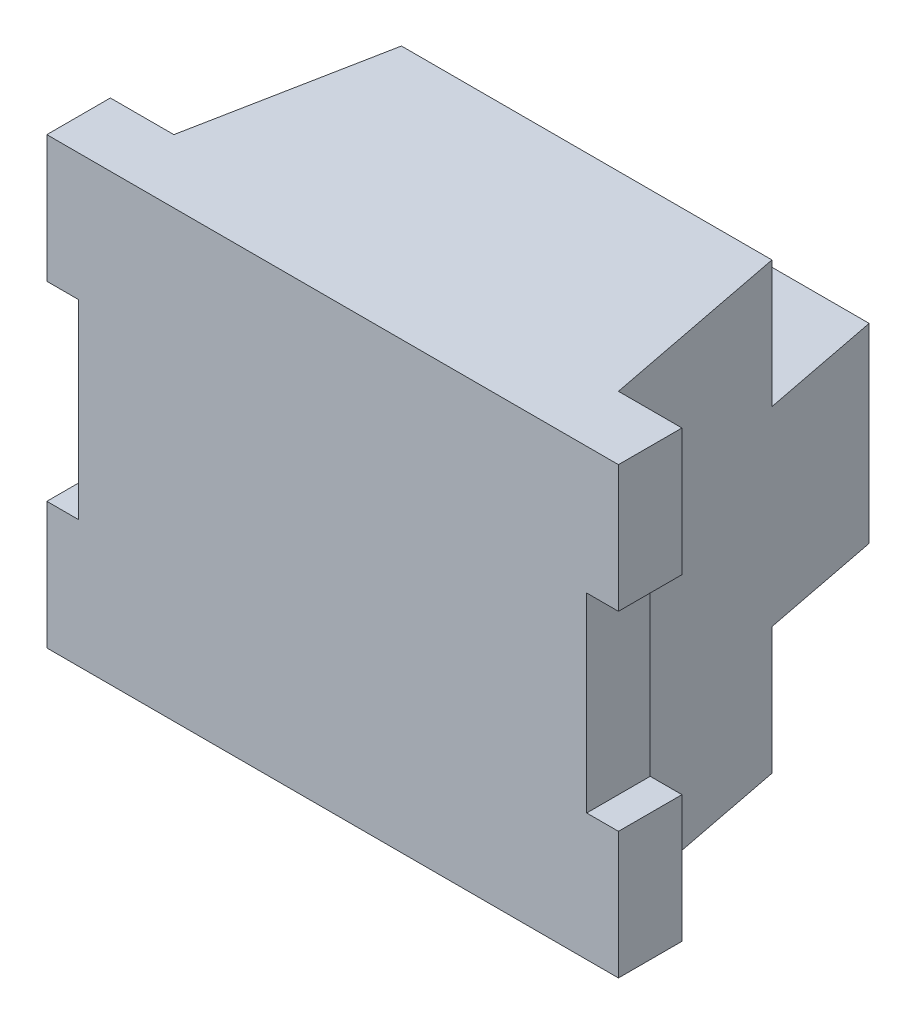
ISO-10303-21;
HEADER;
FILE_DESCRIPTION(('STEP AP214'),'2;1');
FILE_NAME('part.step','',(''),(''),'','','');
FILE_SCHEMA(('AUTOMOTIVE_DESIGN { 1 0 10303 214 1 1 1 1 }'));
ENDSEC;
DATA;
#1=APPLICATION_CONTEXT('core data for automotive mechanical design processes');
#2=APPLICATION_PROTOCOL_DEFINITION('international standard','automotive_design',2000,#1);
#3=PRODUCT_CONTEXT('',#1,'mechanical');
#4=PRODUCT('Part','Part','',(#3));
#5=PRODUCT_RELATED_PRODUCT_CATEGORY('part','',(#4));
#6=PRODUCT_DEFINITION_FORMATION('','',#4);
#7=PRODUCT_DEFINITION_CONTEXT('part definition',#1,'design');
#8=PRODUCT_DEFINITION('design','',#6,#7);
#9=PRODUCT_DEFINITION_SHAPE('','',#8);
#10=(LENGTH_UNIT() NAMED_UNIT(*) SI_UNIT(.MILLI.,.METRE.));
#11=(NAMED_UNIT(*) PLANE_ANGLE_UNIT() SI_UNIT($,.RADIAN.));
#12=(NAMED_UNIT(*) SI_UNIT($,.STERADIAN.) SOLID_ANGLE_UNIT());
#13=UNCERTAINTY_MEASURE_WITH_UNIT(LENGTH_MEASURE(1.E-05),#10,'distance_accuracy_value','');
#14=(GEOMETRIC_REPRESENTATION_CONTEXT(3) GLOBAL_UNCERTAINTY_ASSIGNED_CONTEXT((#13)) GLOBAL_UNIT_ASSIGNED_CONTEXT((#10,
#11,#12)) REPRESENTATION_CONTEXT('',''));
#15=CARTESIAN_POINT('',(0.,0.,0.));
#16=DIRECTION('',(0.,0.,1.));
#17=DIRECTION('',(1.,0.,0.));
#18=AXIS2_PLACEMENT_3D('',#15,#16,#17);
#19=CARTESIAN_POINT('',(-45.,35.,10.));
#20=DIRECTION('',(0.,-1.,0.));
#21=DIRECTION('',(0.,0.,-1.));
#22=AXIS2_PLACEMENT_3D('',#19,#20,#21);
#23=PLANE('',#22);
#24=DIRECTION('',(1.,0.,0.));
#25=VECTOR('',#24,1.);
#26=CARTESIAN_POINT('',(38.9138217050319,35.,-30.));
#27=LINE('',#26,#25);
#28=CARTESIAN_POINT('',(-29.1685907258683,35.,-30.));
#29=VERTEX_POINT('',#28);
#30=CARTESIAN_POINT('',(29.1685907258683,35.,-30.));
#31=VERTEX_POINT('',#30);
#32=EDGE_CURVE('E61',#29,#31,#27,.T.);
#33=ORIENTED_EDGE('',*,*,#32,.F.);
#34=DIRECTION('',(-0.190808995376549,0.,0.981627183447663));
#35=VECTOR('',#34,1.);
#36=CARTESIAN_POINT('',(-25.4753648522516,35.,-49.));
#37=LINE('',#36,#35);
#38=CARTESIAN_POINT('',(-35.,35.,0.));
#39=VERTEX_POINT('',#38);
#40=EDGE_CURVE('E209',#29,#39,#37,.T.);
#41=ORIENTED_EDGE('',*,*,#40,.T.);
#42=DIRECTION('',(-1.,0.,0.));
#43=VECTOR('',#42,1.);
#44=CARTESIAN_POINT('',(-45.,35.,0.));
#45=LINE('',#44,#43);
#46=CARTESIAN_POINT('',(-45.,35.,0.));
#47=VERTEX_POINT('',#46);
#48=EDGE_CURVE('E259',#39,#47,#45,.T.);
#49=ORIENTED_EDGE('',*,*,#48,.T.);
#50=DIRECTION('',(0.,0.,-1.));
#51=VECTOR('',#50,1.);
#52=CARTESIAN_POINT('',(-45.,35.,10.));
#53=LINE('',#52,#51);
#54=CARTESIAN_POINT('',(-45.,35.,10.));
#55=VERTEX_POINT('',#54);
#56=EDGE_CURVE('E291',#55,#47,#53,.T.);
#57=ORIENTED_EDGE('',*,*,#56,.F.);
#58=DIRECTION('',(-1.,0.,0.));
#59=VECTOR('',#58,1.);
#60=CARTESIAN_POINT('',(-45.,35.,10.));
#61=LINE('',#60,#59);
#62=CARTESIAN_POINT('',(45.,35.,10.));
#63=VERTEX_POINT('',#62);
#64=EDGE_CURVE('E234',#63,#55,#61,.T.);
#65=ORIENTED_EDGE('',*,*,#64,.F.);
#66=DIRECTION('',(0.,0.,-1.));
#67=VECTOR('',#66,1.);
#68=CARTESIAN_POINT('',(45.,35.,10.));
#69=LINE('',#68,#67);
#70=CARTESIAN_POINT('',(45.,35.,0.));
#71=VERTEX_POINT('',#70);
#72=EDGE_CURVE('E299',#63,#71,#69,.T.);
#73=ORIENTED_EDGE('',*,*,#72,.T.);
#74=CARTESIAN_POINT('',(35.,35.,0.));
#75=VERTEX_POINT('',#74);
#76=EDGE_CURVE('E257',#71,#75,#45,.T.);
#77=ORIENTED_EDGE('',*,*,#76,.T.);
#78=DIRECTION('',(-0.190808995376549,0.,-0.981627183447663));
#79=VECTOR('',#78,1.);
#80=CARTESIAN_POINT('',(35.,35.,0.));
#81=LINE('',#80,#79);
#82=EDGE_CURVE('E201',#75,#31,#81,.T.);
#83=ORIENTED_EDGE('',*,*,#82,.T.);
#84=EDGE_LOOP('',(#33,#41,#49,#57,#65,#73,#77,#83));
#85=FACE_BOUND('',#84,.T.);
#86=ADVANCED_FACE('F39',(#85),#23,.F.);
#87=CARTESIAN_POINT('',(-45.,-35.,10.));
#88=DIRECTION('',(0.,1.,0.));
#89=DIRECTION('',(0.,0.,1.));
#90=AXIS2_PLACEMENT_3D('',#87,#88,#89);
#91=PLANE('',#90);
#92=DIRECTION('',(-1.,0.,0.));
#93=VECTOR('',#92,1.);
#94=CARTESIAN_POINT('',(38.9138217050319,-35.,-30.));
#95=LINE('',#94,#93);
#96=CARTESIAN_POINT('',(29.1685907258683,-35.,-30.));
#97=VERTEX_POINT('',#96);
#98=CARTESIAN_POINT('',(-29.1685907258683,-35.,-30.));
#99=VERTEX_POINT('',#98);
#100=EDGE_CURVE('E178',#97,#99,#95,.T.);
#101=ORIENTED_EDGE('',*,*,#100,.F.);
#102=DIRECTION('',(0.190808995376549,0.,0.981627183447663));
#103=VECTOR('',#102,1.);
#104=CARTESIAN_POINT('',(35.,-35.,0.));
#105=LINE('',#104,#103);
#106=CARTESIAN_POINT('',(35.,-35.,0.));
#107=VERTEX_POINT('',#106);
#108=EDGE_CURVE('E206',#97,#107,#105,.T.);
#109=ORIENTED_EDGE('',*,*,#108,.T.);
#110=DIRECTION('',(1.,0.,0.));
#111=VECTOR('',#110,1.);
#112=CARTESIAN_POINT('',(-45.,-35.,0.));
#113=LINE('',#112,#111);
#114=CARTESIAN_POINT('',(45.,-35.,0.));
#115=VERTEX_POINT('',#114);
#116=EDGE_CURVE('E272',#107,#115,#113,.T.);
#117=ORIENTED_EDGE('',*,*,#116,.T.);
#118=DIRECTION('',(0.,0.,-1.));
#119=VECTOR('',#118,1.);
#120=CARTESIAN_POINT('',(45.,-35.,10.));
#121=LINE('',#120,#119);
#122=CARTESIAN_POINT('',(45.,-35.,10.));
#123=VERTEX_POINT('',#122);
#124=EDGE_CURVE('E246',#123,#115,#121,.T.);
#125=ORIENTED_EDGE('',*,*,#124,.F.);
#126=DIRECTION('',(1.,0.,0.));
#127=VECTOR('',#126,1.);
#128=CARTESIAN_POINT('',(-45.,-35.,10.));
#129=LINE('',#128,#127);
#130=CARTESIAN_POINT('',(-45.,-35.,10.));
#131=VERTEX_POINT('',#130);
#132=EDGE_CURVE('E248',#131,#123,#129,.T.);
#133=ORIENTED_EDGE('',*,*,#132,.F.);
#134=DIRECTION('',(0.,0.,-1.));
#135=VECTOR('',#134,1.);
#136=CARTESIAN_POINT('',(-45.,-35.,10.));
#137=LINE('',#136,#135);
#138=CARTESIAN_POINT('',(-45.,-35.,0.));
#139=VERTEX_POINT('',#138);
#140=EDGE_CURVE('E279',#131,#139,#137,.T.);
#141=ORIENTED_EDGE('',*,*,#140,.T.);
#142=CARTESIAN_POINT('',(-35.,-35.,0.));
#143=VERTEX_POINT('',#142);
#144=EDGE_CURVE('E229',#139,#143,#113,.T.);
#145=ORIENTED_EDGE('',*,*,#144,.T.);
#146=DIRECTION('',(0.190808995376549,0.,-0.981627183447663));
#147=VECTOR('',#146,1.);
#148=CARTESIAN_POINT('',(-25.4753648522516,-35.,-49.));
#149=LINE('',#148,#147);
#150=EDGE_CURVE('E204',#143,#99,#149,.T.);
#151=ORIENTED_EDGE('',*,*,#150,.T.);
#152=EDGE_LOOP('',(#101,#109,#117,#125,#133,#141,#145,#151));
#153=FACE_BOUND('',#152,.T.);
#154=ADVANCED_FACE('F334',(#153),#91,.F.);
#155=CARTESIAN_POINT('',(0.,0.,0.));
#156=DIRECTION('',(0.,0.,1.));
#157=DIRECTION('',(1.,0.,0.));
#158=AXIS2_PLACEMENT_3D('',#155,#156,#157);
#159=PLANE('',#158);
#160=DIRECTION('',(0.,1.,0.));
#161=VECTOR('',#160,1.);
#162=CARTESIAN_POINT('',(-35.,-120.445889310136,0.));
#163=LINE('',#162,#161);
#164=EDGE_CURVE('E210',#143,#39,#163,.T.);
#165=ORIENTED_EDGE('',*,*,#164,.F.);
#166=ORIENTED_EDGE('',*,*,#144,.F.);
#167=DIRECTION('',(0.,-1.,0.));
#168=VECTOR('',#167,1.);
#169=CARTESIAN_POINT('',(-45.,-15.,0.));
#170=LINE('',#169,#168);
#171=CARTESIAN_POINT('',(-45.,-15.,0.));
#172=VERTEX_POINT('',#171);
#173=EDGE_CURVE('E271',#172,#139,#170,.T.);
#174=ORIENTED_EDGE('',*,*,#173,.F.);
#175=DIRECTION('',(-1.,0.,0.));
#176=VECTOR('',#175,1.);
#177=CARTESIAN_POINT('',(-45.,-15.,0.));
#178=LINE('',#177,#176);
#179=CARTESIAN_POINT('',(-40.,-15.,0.));
#180=VERTEX_POINT('',#179);
#181=EDGE_CURVE('E267',#180,#172,#178,.T.);
#182=ORIENTED_EDGE('',*,*,#181,.F.);
#183=DIRECTION('',(0.,-1.,0.));
#184=VECTOR('',#183,1.);
#185=CARTESIAN_POINT('',(-40.,15.,0.));
#186=LINE('',#185,#184);
#187=CARTESIAN_POINT('',(-40.,15.,0.));
#188=VERTEX_POINT('',#187);
#189=EDGE_CURVE('E270',#188,#180,#186,.T.);
#190=ORIENTED_EDGE('',*,*,#189,.F.);
#191=DIRECTION('',(1.,0.,0.));
#192=VECTOR('',#191,1.);
#193=CARTESIAN_POINT('',(-45.,15.,0.));
#194=LINE('',#193,#192);
#195=CARTESIAN_POINT('',(-45.,15.,0.));
#196=VERTEX_POINT('',#195);
#197=EDGE_CURVE('E264',#196,#188,#194,.T.);
#198=ORIENTED_EDGE('',*,*,#197,.F.);
#199=DIRECTION('',(0.,-1.,0.));
#200=VECTOR('',#199,1.);
#201=CARTESIAN_POINT('',(-45.,35.,0.));
#202=LINE('',#201,#200);
#203=EDGE_CURVE('E263',#47,#196,#202,.T.);
#204=ORIENTED_EDGE('',*,*,#203,.F.);
#205=ORIENTED_EDGE('',*,*,#48,.F.);
#206=EDGE_LOOP('',(#165,#166,#174,#182,#190,#198,#204,#205));
#207=FACE_BOUND('',#206,.T.);
#208=ADVANCED_FACE('F346',(#207),#159,.F.);
#209=CARTESIAN_POINT('',(45.,-15.,10.));
#210=DIRECTION('',(-1.,0.,0.));
#211=DIRECTION('',(0.,-1.,0.));
#212=AXIS2_PLACEMENT_3D('',#209,#210,#211);
#213=PLANE('',#212);
#214=DIRECTION('',(0.,1.,0.));
#215=VECTOR('',#214,1.);
#216=CARTESIAN_POINT('',(45.,-15.,0.));
#217=LINE('',#216,#215);
#218=CARTESIAN_POINT('',(45.,-15.,0.));
#219=VERTEX_POINT('',#218);
#220=EDGE_CURVE('E222',#115,#219,#217,.T.);
#221=ORIENTED_EDGE('',*,*,#220,.T.);
#222=DIRECTION('',(0.,0.,-1.));
#223=VECTOR('',#222,1.);
#224=CARTESIAN_POINT('',(45.,-15.,10.));
#225=LINE('',#224,#223);
#226=CARTESIAN_POINT('',(45.,-15.,10.));
#227=VERTEX_POINT('',#226);
#228=EDGE_CURVE('E306',#227,#219,#225,.T.);
#229=ORIENTED_EDGE('',*,*,#228,.F.);
#230=DIRECTION('',(0.,1.,0.));
#231=VECTOR('',#230,1.);
#232=CARTESIAN_POINT('',(45.,-15.,10.));
#233=LINE('',#232,#231);
#234=EDGE_CURVE('E225',#123,#227,#233,.T.);
#235=ORIENTED_EDGE('',*,*,#234,.F.);
#236=ORIENTED_EDGE('',*,*,#124,.T.);
#237=EDGE_LOOP('',(#221,#229,#235,#236));
#238=FACE_BOUND('',#237,.T.);
#239=ADVANCED_FACE('F41',(#238),#213,.F.);
#240=CARTESIAN_POINT('',(45.,-15.,10.));
#241=DIRECTION('',(0.,-1.,0.));
#242=DIRECTION('',(1.,0.,0.));
#243=AXIS2_PLACEMENT_3D('',#240,#241,#242);
#244=PLANE('',#243);
#245=DIRECTION('',(-1.,0.,0.));
#246=VECTOR('',#245,1.);
#247=CARTESIAN_POINT('',(45.,-15.,0.));
#248=LINE('',#247,#246);
#249=CARTESIAN_POINT('',(40.,-15.,0.));
#250=VERTEX_POINT('',#249);
#251=EDGE_CURVE('E253',#219,#250,#248,.T.);
#252=ORIENTED_EDGE('',*,*,#251,.T.);
#253=DIRECTION('',(0.,0.,-1.));
#254=VECTOR('',#253,1.);
#255=CARTESIAN_POINT('',(40.,-15.,10.));
#256=LINE('',#255,#254);
#257=CARTESIAN_POINT('',(40.,-15.,10.));
#258=VERTEX_POINT('',#257);
#259=EDGE_CURVE('E302',#258,#250,#256,.T.);
#260=ORIENTED_EDGE('',*,*,#259,.F.);
#261=DIRECTION('',(-1.,0.,0.));
#262=VECTOR('',#261,1.);
#263=CARTESIAN_POINT('',(45.,-15.,10.));
#264=LINE('',#263,#262);
#265=EDGE_CURVE('E223',#227,#258,#264,.T.);
#266=ORIENTED_EDGE('',*,*,#265,.F.);
#267=ORIENTED_EDGE('',*,*,#228,.T.);
#268=EDGE_LOOP('',(#252,#260,#266,#267));
#269=FACE_BOUND('',#268,.T.);
#270=ADVANCED_FACE('F378',(#269),#244,.F.);
#271=CARTESIAN_POINT('',(40.,15.,10.));
#272=DIRECTION('',(-1.,0.,0.));
#273=DIRECTION('',(0.,0.,1.));
#274=AXIS2_PLACEMENT_3D('',#271,#272,#273);
#275=PLANE('',#274);
#276=DIRECTION('',(0.,1.,0.));
#277=VECTOR('',#276,1.);
#278=CARTESIAN_POINT('',(40.,15.,0.));
#279=LINE('',#278,#277);
#280=CARTESIAN_POINT('',(40.,15.,0.));
#281=VERTEX_POINT('',#280);
#282=EDGE_CURVE('E251',#250,#281,#279,.T.);
#283=ORIENTED_EDGE('',*,*,#282,.T.);
#284=DIRECTION('',(0.,0.,-1.));
#285=VECTOR('',#284,1.);
#286=CARTESIAN_POINT('',(40.,15.,10.));
#287=LINE('',#286,#285);
#288=CARTESIAN_POINT('',(40.,15.,10.));
#289=VERTEX_POINT('',#288);
#290=EDGE_CURVE('E305',#289,#281,#287,.T.);
#291=ORIENTED_EDGE('',*,*,#290,.F.);
#292=DIRECTION('',(0.,1.,0.));
#293=VECTOR('',#292,1.);
#294=CARTESIAN_POINT('',(40.,15.,10.));
#295=LINE('',#294,#293);
#296=EDGE_CURVE('E230',#258,#289,#295,.T.);
#297=ORIENTED_EDGE('',*,*,#296,.F.);
#298=ORIENTED_EDGE('',*,*,#259,.T.);
#299=EDGE_LOOP('',(#283,#291,#297,#298));
#300=FACE_BOUND('',#299,.T.);
#301=ADVANCED_FACE('F372',(#300),#275,.F.);
#302=CARTESIAN_POINT('',(45.,15.,10.));
#303=DIRECTION('',(0.,1.,0.));
#304=DIRECTION('',(0.,0.,1.));
#305=AXIS2_PLACEMENT_3D('',#302,#303,#304);
#306=PLANE('',#305);
#307=DIRECTION('',(1.,0.,0.));
#308=VECTOR('',#307,1.);
#309=CARTESIAN_POINT('',(45.,15.,0.));
#310=LINE('',#309,#308);
#311=CARTESIAN_POINT('',(45.,15.,0.));
#312=VERTEX_POINT('',#311);
#313=EDGE_CURVE('E254',#281,#312,#310,.T.);
#314=ORIENTED_EDGE('',*,*,#313,.T.);
#315=DIRECTION('',(0.,0.,-1.));
#316=VECTOR('',#315,1.);
#317=CARTESIAN_POINT('',(45.,15.,10.));
#318=LINE('',#317,#316);
#319=CARTESIAN_POINT('',(45.,15.,10.));
#320=VERTEX_POINT('',#319);
#321=EDGE_CURVE('E298',#320,#312,#318,.T.);
#322=ORIENTED_EDGE('',*,*,#321,.F.);
#323=DIRECTION('',(1.,0.,0.));
#324=VECTOR('',#323,1.);
#325=CARTESIAN_POINT('',(45.,15.,10.));
#326=LINE('',#325,#324);
#327=EDGE_CURVE('E227',#289,#320,#326,.T.);
#328=ORIENTED_EDGE('',*,*,#327,.F.);
#329=ORIENTED_EDGE('',*,*,#290,.T.);
#330=EDGE_LOOP('',(#314,#322,#328,#329));
#331=FACE_BOUND('',#330,.T.);
#332=ADVANCED_FACE('F367',(#331),#306,.F.);
#333=CARTESIAN_POINT('',(45.,35.,10.));
#334=DIRECTION('',(-1.,0.,0.));
#335=DIRECTION('',(0.,-1.,0.));
#336=AXIS2_PLACEMENT_3D('',#333,#334,#335);
#337=PLANE('',#336);
#338=DIRECTION('',(0.,1.,0.));
#339=VECTOR('',#338,1.);
#340=CARTESIAN_POINT('',(45.,35.,0.));
#341=LINE('',#340,#339);
#342=EDGE_CURVE('E260',#312,#71,#341,.T.);
#343=ORIENTED_EDGE('',*,*,#342,.T.);
#344=ORIENTED_EDGE('',*,*,#72,.F.);
#345=DIRECTION('',(0.,1.,0.));
#346=VECTOR('',#345,1.);
#347=CARTESIAN_POINT('',(45.,35.,10.));
#348=LINE('',#347,#346);
#349=EDGE_CURVE('E235',#320,#63,#348,.T.);
#350=ORIENTED_EDGE('',*,*,#349,.F.);
#351=ORIENTED_EDGE('',*,*,#321,.T.);
#352=EDGE_LOOP('',(#343,#344,#350,#351));
#353=FACE_BOUND('',#352,.T.);
#354=ADVANCED_FACE('F366',(#353),#337,.F.);
#355=CARTESIAN_POINT('',(-45.,35.,10.));
#356=DIRECTION('',(1.,0.,0.));
#357=DIRECTION('',(0.,1.,0.));
#358=AXIS2_PLACEMENT_3D('',#355,#356,#357);
#359=PLANE('',#358);
#360=ORIENTED_EDGE('',*,*,#203,.T.);
#361=DIRECTION('',(0.,0.,-1.));
#362=VECTOR('',#361,1.);
#363=CARTESIAN_POINT('',(-45.,15.,10.));
#364=LINE('',#363,#362);
#365=CARTESIAN_POINT('',(-45.,15.,10.));
#366=VERTEX_POINT('',#365);
#367=EDGE_CURVE('E287',#366,#196,#364,.T.);
#368=ORIENTED_EDGE('',*,*,#367,.F.);
#369=DIRECTION('',(0.,-1.,0.));
#370=VECTOR('',#369,1.);
#371=CARTESIAN_POINT('',(-45.,35.,10.));
#372=LINE('',#371,#370);
#373=EDGE_CURVE('E237',#55,#366,#372,.T.);
#374=ORIENTED_EDGE('',*,*,#373,.F.);
#375=ORIENTED_EDGE('',*,*,#56,.T.);
#376=EDGE_LOOP('',(#360,#368,#374,#375));
#377=FACE_BOUND('',#376,.T.);
#378=ADVANCED_FACE('F353',(#377),#359,.F.);
#379=CARTESIAN_POINT('',(-45.,15.,10.));
#380=DIRECTION('',(0.,1.,0.));
#381=DIRECTION('',(0.,0.,1.));
#382=AXIS2_PLACEMENT_3D('',#379,#380,#381);
#383=PLANE('',#382);
#384=ORIENTED_EDGE('',*,*,#197,.T.);
#385=DIRECTION('',(0.,0.,-1.));
#386=VECTOR('',#385,1.);
#387=CARTESIAN_POINT('',(-40.,15.,10.));
#388=LINE('',#387,#386);
#389=CARTESIAN_POINT('',(-40.,15.,10.));
#390=VERTEX_POINT('',#389);
#391=EDGE_CURVE('E290',#390,#188,#388,.T.);
#392=ORIENTED_EDGE('',*,*,#391,.F.);
#393=DIRECTION('',(1.,0.,0.));
#394=VECTOR('',#393,1.);
#395=CARTESIAN_POINT('',(-45.,15.,10.));
#396=LINE('',#395,#394);
#397=EDGE_CURVE('E236',#366,#390,#396,.T.);
#398=ORIENTED_EDGE('',*,*,#397,.F.);
#399=ORIENTED_EDGE('',*,*,#367,.T.);
#400=EDGE_LOOP('',(#384,#392,#398,#399));
#401=FACE_BOUND('',#400,.T.);
#402=ADVANCED_FACE('F356',(#401),#383,.F.);
#403=CARTESIAN_POINT('',(-40.,15.,10.));
#404=DIRECTION('',(1.,0.,0.));
#405=DIRECTION('',(0.,0.,-1.));
#406=AXIS2_PLACEMENT_3D('',#403,#404,#405);
#407=PLANE('',#406);
#408=ORIENTED_EDGE('',*,*,#189,.T.);
#409=DIRECTION('',(0.,0.,-1.));
#410=VECTOR('',#409,1.);
#411=CARTESIAN_POINT('',(-40.,-15.,10.));
#412=LINE('',#411,#410);
#413=CARTESIAN_POINT('',(-40.,-15.,10.));
#414=VERTEX_POINT('',#413);
#415=EDGE_CURVE('E283',#414,#180,#412,.T.);
#416=ORIENTED_EDGE('',*,*,#415,.F.);
#417=DIRECTION('',(0.,-1.,0.));
#418=VECTOR('',#417,1.);
#419=CARTESIAN_POINT('',(-40.,15.,10.));
#420=LINE('',#419,#418);
#421=EDGE_CURVE('E238',#390,#414,#420,.T.);
#422=ORIENTED_EDGE('',*,*,#421,.F.);
#423=ORIENTED_EDGE('',*,*,#391,.T.);
#424=EDGE_LOOP('',(#408,#416,#422,#423));
#425=FACE_BOUND('',#424,.T.);
#426=ADVANCED_FACE('F393',(#425),#407,.F.);
#427=CARTESIAN_POINT('',(-45.,-15.,10.));
#428=DIRECTION('',(0.,-1.,0.));
#429=DIRECTION('',(0.,0.,-1.));
#430=AXIS2_PLACEMENT_3D('',#427,#428,#429);
#431=PLANE('',#430);
#432=ORIENTED_EDGE('',*,*,#181,.T.);
#433=DIRECTION('',(0.,0.,-1.));
#434=VECTOR('',#433,1.);
#435=CARTESIAN_POINT('',(-45.,-15.,10.));
#436=LINE('',#435,#434);
#437=CARTESIAN_POINT('',(-45.,-15.,10.));
#438=VERTEX_POINT('',#437);
#439=EDGE_CURVE('E284',#438,#172,#436,.T.);
#440=ORIENTED_EDGE('',*,*,#439,.F.);
#441=DIRECTION('',(-1.,0.,0.));
#442=VECTOR('',#441,1.);
#443=CARTESIAN_POINT('',(-45.,-15.,10.));
#444=LINE('',#443,#442);
#445=EDGE_CURVE('E241',#414,#438,#444,.T.);
#446=ORIENTED_EDGE('',*,*,#445,.F.);
#447=ORIENTED_EDGE('',*,*,#415,.T.);
#448=EDGE_LOOP('',(#432,#440,#446,#447));
#449=FACE_BOUND('',#448,.T.);
#450=ADVANCED_FACE('F391',(#449),#431,.F.);
#451=CARTESIAN_POINT('',(-45.,-15.,10.));
#452=DIRECTION('',(1.,0.,0.));
#453=DIRECTION('',(0.,1.,0.));
#454=AXIS2_PLACEMENT_3D('',#451,#452,#453);
#455=PLANE('',#454);
#456=ORIENTED_EDGE('',*,*,#173,.T.);
#457=ORIENTED_EDGE('',*,*,#140,.F.);
#458=DIRECTION('',(0.,-1.,0.));
#459=VECTOR('',#458,1.);
#460=CARTESIAN_POINT('',(-45.,-15.,10.));
#461=LINE('',#460,#459);
#462=EDGE_CURVE('E243',#438,#131,#461,.T.);
#463=ORIENTED_EDGE('',*,*,#462,.F.);
#464=ORIENTED_EDGE('',*,*,#439,.T.);
#465=EDGE_LOOP('',(#456,#457,#463,#464));
#466=FACE_BOUND('',#465,.T.);
#467=ADVANCED_FACE('F389',(#466),#455,.F.);
#468=CARTESIAN_POINT('',(0.,0.,10.));
#469=DIRECTION('',(0.,0.,1.));
#470=DIRECTION('',(1.,0.,0.));
#471=AXIS2_PLACEMENT_3D('',#468,#469,#470);
#472=PLANE('',#471);
#473=ORIENTED_EDGE('',*,*,#234,.T.);
#474=ORIENTED_EDGE('',*,*,#265,.T.);
#475=ORIENTED_EDGE('',*,*,#296,.T.);
#476=ORIENTED_EDGE('',*,*,#327,.T.);
#477=ORIENTED_EDGE('',*,*,#349,.T.);
#478=ORIENTED_EDGE('',*,*,#64,.T.);
#479=ORIENTED_EDGE('',*,*,#373,.T.);
#480=ORIENTED_EDGE('',*,*,#397,.T.);
#481=ORIENTED_EDGE('',*,*,#421,.T.);
#482=ORIENTED_EDGE('',*,*,#445,.T.);
#483=ORIENTED_EDGE('',*,*,#462,.T.);
#484=ORIENTED_EDGE('',*,*,#132,.T.);
#485=EDGE_LOOP('',(#473,#474,#475,#476,#477,#478,#479,#480,#481,#482,#483,#484));
#486=FACE_BOUND('',#485,.T.);
#487=ADVANCED_FACE('F362',(#486),#472,.T.);
#488=ORIENTED_EDGE('',*,*,#116,.F.);
#489=DIRECTION('',(0.,1.,0.));
#490=VECTOR('',#489,1.);
#491=CARTESIAN_POINT('',(35.,-120.445889310136,0.));
#492=LINE('',#491,#490);
#493=EDGE_CURVE('E215',#107,#75,#492,.T.);
#494=ORIENTED_EDGE('',*,*,#493,.T.);
#495=ORIENTED_EDGE('',*,*,#76,.F.);
#496=ORIENTED_EDGE('',*,*,#342,.F.);
#497=ORIENTED_EDGE('',*,*,#313,.F.);
#498=ORIENTED_EDGE('',*,*,#282,.F.);
#499=ORIENTED_EDGE('',*,*,#251,.F.);
#500=ORIENTED_EDGE('',*,*,#220,.F.);
#501=EDGE_LOOP('',(#488,#494,#495,#496,#497,#498,#499,#500));
#502=FACE_BOUND('',#501,.T.);
#503=ADVANCED_FACE('F327',(#502),#159,.F.);
#504=CARTESIAN_POINT('',(-25.4753648522516,-120.445889310136,-49.));
#505=DIRECTION('',(-0.981627183447663,0.,-0.190808995376549));
#506=DIRECTION('',(-0.190808995376549,0.,0.981627183447663));
#507=AXIS2_PLACEMENT_3D('',#504,#505,#506);
#508=PLANE('',#507);
#509=DIRECTION('',(-0.190808995376549,0.,0.981627183447663));
#510=VECTOR('',#509,1.);
#511=CARTESIAN_POINT('',(-25.4753648522516,15.,-49.));
#512=LINE('',#511,#510);
#513=CARTESIAN_POINT('',(-25.4753648522516,15.,-49.));
#514=VERTEX_POINT('',#513);
#515=CARTESIAN_POINT('',(-29.1685907258683,15.,-30.));
#516=VERTEX_POINT('',#515);
#517=EDGE_CURVE('E196',#514,#516,#512,.T.);
#518=ORIENTED_EDGE('',*,*,#517,.F.);
#519=DIRECTION('',(0.,1.,0.));
#520=VECTOR('',#519,1.);
#521=CARTESIAN_POINT('',(-25.4753648522516,-120.445889310136,-49.));
#522=LINE('',#521,#520);
#523=CARTESIAN_POINT('',(-25.4753648522516,-15.,-49.));
#524=VERTEX_POINT('',#523);
#525=EDGE_CURVE('E194',#524,#514,#522,.T.);
#526=ORIENTED_EDGE('',*,*,#525,.F.);
#527=DIRECTION('',(0.190808995376549,0.,-0.981627183447663));
#528=VECTOR('',#527,1.);
#529=CARTESIAN_POINT('',(-25.4753648522516,-15.,-49.));
#530=LINE('',#529,#528);
#531=CARTESIAN_POINT('',(-29.1685907258683,-15.,-30.));
#532=VERTEX_POINT('',#531);
#533=EDGE_CURVE('E182',#532,#524,#530,.T.);
#534=ORIENTED_EDGE('',*,*,#533,.F.);
#535=DIRECTION('',(0.,1.,0.));
#536=VECTOR('',#535,1.);
#537=CARTESIAN_POINT('',(-29.1685907258683,-120.445889310136,-30.));
#538=LINE('',#537,#536);
#539=EDGE_CURVE('E175',#99,#532,#538,.T.);
#540=ORIENTED_EDGE('',*,*,#539,.F.);
#541=ORIENTED_EDGE('',*,*,#150,.F.);
#542=ORIENTED_EDGE('',*,*,#164,.T.);
#543=ORIENTED_EDGE('',*,*,#40,.F.);
#544=DIRECTION('',(0.,-1.,0.));
#545=VECTOR('',#544,1.);
#546=CARTESIAN_POINT('',(-29.1685907258683,-120.445889310136,-30.));
#547=LINE('',#546,#545);
#548=EDGE_CURVE('E192',#29,#516,#547,.T.);
#549=ORIENTED_EDGE('',*,*,#548,.T.);
#550=EDGE_LOOP('',(#518,#526,#534,#540,#541,#542,#543,#549));
#551=FACE_BOUND('',#550,.T.);
#552=ADVANCED_FACE('F195',(#551),#508,.T.);
#553=CARTESIAN_POINT('',(-25.4753648522516,-120.445889310136,-49.));
#554=DIRECTION('',(0.,0.,-1.));
#555=DIRECTION('',(-1.,0.,0.));
#556=AXIS2_PLACEMENT_3D('',#553,#554,#555);
#557=PLANE('',#556);
#558=DIRECTION('',(-1.,0.,0.));
#559=VECTOR('',#558,1.);
#560=CARTESIAN_POINT('',(38.9138217050319,15.,-49.));
#561=LINE('',#560,#559);
#562=CARTESIAN_POINT('',(25.4753648522516,15.,-49.));
#563=VERTEX_POINT('',#562);
#564=EDGE_CURVE('E339',#563,#514,#561,.T.);
#565=ORIENTED_EDGE('',*,*,#564,.F.);
#566=DIRECTION('',(0.,1.,0.));
#567=VECTOR('',#566,1.);
#568=CARTESIAN_POINT('',(25.4753648522516,-120.445889310136,-49.));
#569=LINE('',#568,#567);
#570=CARTESIAN_POINT('',(25.4753648522516,-15.,-49.));
#571=VERTEX_POINT('',#570);
#572=EDGE_CURVE('E216',#571,#563,#569,.T.);
#573=ORIENTED_EDGE('',*,*,#572,.F.);
#574=DIRECTION('',(1.,0.,0.));
#575=VECTOR('',#574,1.);
#576=CARTESIAN_POINT('',(38.9138217050319,-15.,-49.));
#577=LINE('',#576,#575);
#578=EDGE_CURVE('E333',#524,#571,#577,.T.);
#579=ORIENTED_EDGE('',*,*,#578,.F.);
#580=ORIENTED_EDGE('',*,*,#525,.T.);
#581=EDGE_LOOP('',(#565,#573,#579,#580));
#582=FACE_BOUND('',#581,.T.);
#583=ADVANCED_FACE('F435',(#582),#557,.T.);
#584=CARTESIAN_POINT('',(35.,-120.445889310136,0.));
#585=DIRECTION('',(0.981627183447663,0.,-0.190808995376549));
#586=DIRECTION('',(-0.190808995376549,0.,-0.981627183447663));
#587=AXIS2_PLACEMENT_3D('',#584,#585,#586);
#588=PLANE('',#587);
#589=DIRECTION('',(-0.190808995376549,0.,-0.981627183447663));
#590=VECTOR('',#589,1.);
#591=CARTESIAN_POINT('',(35.,15.,0.));
#592=LINE('',#591,#590);
#593=CARTESIAN_POINT('',(29.1685907258683,15.,-30.));
#594=VERTEX_POINT('',#593);
#595=EDGE_CURVE('E11',#594,#563,#592,.T.);
#596=ORIENTED_EDGE('',*,*,#595,.F.);
#597=DIRECTION('',(0.,1.,0.));
#598=VECTOR('',#597,1.);
#599=CARTESIAN_POINT('',(29.1685907258683,-120.445889310136,-30.));
#600=LINE('',#599,#598);
#601=EDGE_CURVE('E50',#594,#31,#600,.T.);
#602=ORIENTED_EDGE('',*,*,#601,.T.);
#603=ORIENTED_EDGE('',*,*,#82,.F.);
#604=ORIENTED_EDGE('',*,*,#493,.F.);
#605=ORIENTED_EDGE('',*,*,#108,.F.);
#606=DIRECTION('',(0.,-1.,0.));
#607=VECTOR('',#606,1.);
#608=CARTESIAN_POINT('',(29.1685907258683,-120.445889310136,-30.));
#609=LINE('',#608,#607);
#610=CARTESIAN_POINT('',(29.1685907258683,-15.,-30.));
#611=VERTEX_POINT('',#610);
#612=EDGE_CURVE('E313',#611,#97,#609,.T.);
#613=ORIENTED_EDGE('',*,*,#612,.F.);
#614=DIRECTION('',(0.190808995376549,0.,0.981627183447663));
#615=VECTOR('',#614,1.);
#616=CARTESIAN_POINT('',(35.,-15.,0.));
#617=LINE('',#616,#615);
#618=EDGE_CURVE('E186',#571,#611,#617,.T.);
#619=ORIENTED_EDGE('',*,*,#618,.F.);
#620=ORIENTED_EDGE('',*,*,#572,.T.);
#621=EDGE_LOOP('',(#596,#602,#603,#604,#605,#613,#619,#620));
#622=FACE_BOUND('',#621,.T.);
#623=ADVANCED_FACE('F316',(#622),#588,.T.);
#624=CARTESIAN_POINT('',(38.9138217050319,-15.,-30.));
#625=DIRECTION('',(0.,1.,0.));
#626=DIRECTION('',(0.,0.,1.));
#627=AXIS2_PLACEMENT_3D('',#624,#625,#626);
#628=PLANE('',#627);
#629=ORIENTED_EDGE('',*,*,#533,.T.);
#630=ORIENTED_EDGE('',*,*,#578,.T.);
#631=ORIENTED_EDGE('',*,*,#618,.T.);
#632=DIRECTION('',(1.,0.,0.));
#633=VECTOR('',#632,1.);
#634=CARTESIAN_POINT('',(38.9138217050319,-15.,-30.));
#635=LINE('',#634,#633);
#636=EDGE_CURVE('E53',#532,#611,#635,.T.);
#637=ORIENTED_EDGE('',*,*,#636,.F.);
#638=EDGE_LOOP('',(#629,#630,#631,#637));
#639=FACE_BOUND('',#638,.T.);
#640=ADVANCED_FACE('F184',(#639),#628,.F.);
#641=CARTESIAN_POINT('',(0.,0.,-30.));
#642=DIRECTION('',(0.,0.,1.));
#643=DIRECTION('',(1.,0.,0.));
#644=AXIS2_PLACEMENT_3D('',#641,#642,#643);
#645=PLANE('',#644);
#646=ORIENTED_EDGE('',*,*,#539,.T.);
#647=ORIENTED_EDGE('',*,*,#636,.T.);
#648=ORIENTED_EDGE('',*,*,#612,.T.);
#649=ORIENTED_EDGE('',*,*,#100,.T.);
#650=EDGE_LOOP('',(#646,#647,#648,#649));
#651=FACE_BOUND('',#650,.T.);
#652=ADVANCED_FACE('F173',(#651),#645,.F.);
#653=CARTESIAN_POINT('',(38.9138217050319,15.,-30.));
#654=DIRECTION('',(0.,-1.,0.));
#655=DIRECTION('',(0.,0.,-1.));
#656=AXIS2_PLACEMENT_3D('',#653,#654,#655);
#657=PLANE('',#656);
#658=ORIENTED_EDGE('',*,*,#517,.T.);
#659=DIRECTION('',(-1.,0.,0.));
#660=VECTOR('',#659,1.);
#661=CARTESIAN_POINT('',(38.9138217050319,15.,-30.));
#662=LINE('',#661,#660);
#663=EDGE_CURVE('E337',#594,#516,#662,.T.);
#664=ORIENTED_EDGE('',*,*,#663,.F.);
#665=ORIENTED_EDGE('',*,*,#595,.T.);
#666=ORIENTED_EDGE('',*,*,#564,.T.);
#667=EDGE_LOOP('',(#658,#664,#665,#666));
#668=FACE_BOUND('',#667,.T.);
#669=ADVANCED_FACE('F449',(#668),#657,.F.);
#670=CARTESIAN_POINT('',(0.,0.,-30.));
#671=DIRECTION('',(0.,0.,-1.));
#672=DIRECTION('',(-1.,0.,0.));
#673=AXIS2_PLACEMENT_3D('',#670,#671,#672);
#674=PLANE('',#673);
#675=ORIENTED_EDGE('',*,*,#32,.T.);
#676=ORIENTED_EDGE('',*,*,#601,.F.);
#677=ORIENTED_EDGE('',*,*,#663,.T.);
#678=ORIENTED_EDGE('',*,*,#548,.F.);
#679=EDGE_LOOP('',(#675,#676,#677,#678));
#680=FACE_BOUND('',#679,.T.);
#681=ADVANCED_FACE('F345',(#680),#674,.T.);
#682=CLOSED_SHELL('',(#86,#154,#208,#239,#270,#301,#332,#354,#378,#402,#426,#450,#467,#487,#503,
#552,#583,#623,#640,#652,#669,#681));
#683=MANIFOLD_SOLID_BREP('B2',#682);
#684=ADVANCED_BREP_SHAPE_REPRESENTATION('',(#18,#683),#14);
#685=SHAPE_DEFINITION_REPRESENTATION(#9,#684);
ENDSEC;
END-ISO-10303-21;
